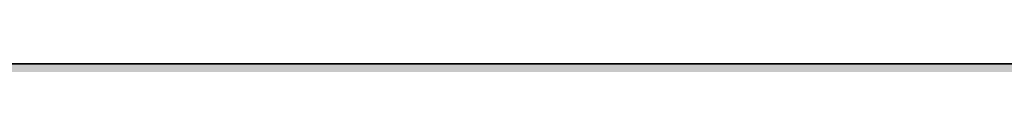
# Model space of a CAD drawing. Units: inches. Extents: x 2091 to 2899, y 967 to 2217.
# Tile 83 of 256: x 2249.731 to 2251.243, y 1099.919 to 1099.919. Entities that reach past the tile are written whole.
import ezdxf

# ---------------------------------------------------------------- set-up
doc = ezdxf.new("R2010")
doc.units = ezdxf.units.IN
doc.layers.add('A-WALL-PATT', color=141, linetype='Continuous', lineweight=13, true_color=0xadddf7)
doc.layers.add('L-SITE-WALL', color=7, linetype='Continuous', lineweight=35)

msp = doc.modelspace()

# ---------------------------------------------------------------- hatches: boundary and pattern name
at = {"layer": 'A-WALL-PATT'}
h = msp.add_hatch(color=256, dxfattribs=at)
h.dxf.hatch_style = 1
h.paths.add_polyline_path([(2212.1436, 1941.4191), (2387.6436, 1941.4191), (2387.6436, 1824.4191), (2392.1436, 1824.4191), (2392.1436, 1941.4191), (2609.6436, 1941.4191), (2609.6436, 1825.9191), (2614.1436, 1825.9191), (2614.1436, 1941.4191), (2794.1436, 1941.4191), (2794.1436, 1928.7622), (2803.1436, 1928.7622), (2803.1436, 2050.9191), (2203.1436, 2050.9191), (2203.1436, 1900.7579), (2212.1436, 1900.7579)])
h.paths.add_polyline_path([(2212.1436, 1945.9191), (2212.1436, 2041.9191), (2794.1436, 2041.9191), (2794.1436, 1945.9191), (2402.2482, 1945.9191), (2401.1024, 1945.7758), (2398.7024, 1945.7758)], flags=16)
h.paths.add_polyline_path([(2230.2299, 1948.0628), (2227.3499, 1949.5028), (2225.9099, 1951.9028), (2223.9899, 1952.8628), (2223.0299, 1955.2628), (2222.0699, 1959.5828), (2222.0699, 1963.4228), (2223.0299, 1965.6628), (2223.9899, 1965.3428), (2225.5859, 1963.8607), (2226.9115, 1964.9573), (2226.9489, 1965.9388), (2227.7783, 1966.9521), (2228.1999, 1968.8787), (2230.7099, 1964.8628), (2233.5899, 1966.3028), (2233.6073, 1966.3319), (2233.7727, 1964.9382), (2234.6338, 1963.6765), (2235.0299, 1963.9028), (2236.282, 1965.5724), (2235.9899, 1962.9428), (2237.9545, 1957.54), (2238.3899, 1957.9028), (2239.2159, 1960.3058), (2238.6546, 1966.385), (2238.6928, 1966.4381), (2238.8406, 1967.4997), (2238.7803, 1967.6875), (2238.8805, 1967.7868), (2238.6669, 1966.2518), (2239.2159, 1960.3058), (2238.3899, 1957.9028), (2236.9499, 1956.7028), (2234.5499, 1949.9828)], flags=0)
h.paths.add_polyline_path([(2278.012, 1948.0628), (2276.4964, 1947.8733), (2275.8498, 1947.6886), (2274.652, 1947.1028)], flags=0)
h.paths.add_polyline_path([(2269.852, 1955.7428), (2268.2762, 1956.6293), (2270.8673, 1956.3484), (2269.372, 1958.1428), (2268.715, 1959.1923), (2270.5698, 1958.7286), (2268.5807, 1961.9061), (2270.812, 1960.8919), (2270.812, 1963.4228), (2271.3933, 1964.7793), (2270.2918, 1966.1562), (2271.772, 1965.6628), (2272.1414, 1966.5248), (2273.9298, 1965.9286), (2275.6304, 1968.0543), (2276.3319, 1966.7219), (2276.5204, 1966.9521), (2276.942, 1968.8787), (2277.7343, 1967.6111), (2278.1399, 1969.4645), (2279.6591, 1967.0337), (2280.412, 1966.7828), (2280.9493, 1967.5888), (2281.6098, 1967.3686), (2282.1333, 1968.1538), (2282.3492, 1966.3334), (2282.3498, 1966.3326), (2283.4076, 1968.0954), (2283.7126, 1965.524), (2284.3202, 1964.6338), (2284.5118, 1964.8892), (2284.235, 1965.7048), (2284.5005, 1967.319), (2284.9079, 1965.4174), (2285.3963, 1966.0686), (2285.4328, 1966.2906), (2285.4733, 1966.1713), (2286.3539, 1967.3454), (2286.222, 1966.1582), (2287.6635, 1968.0802), (2287.714, 1968.4428), (2288.4816, 1969.0167), (2288.574, 1968.7289), (2288.9175, 1969.069), (2288.6068, 1966.8376), (2288.9287, 1963.3513), (2288.935, 1963.3568), (2288.9297, 1963.3404), (2289.0153, 1962.4139), (2290.1112, 1963.8751), (2290.1328, 1963.9426), (2290.2177, 1964.0171), (2290.1112, 1963.8751), (2289.1558, 1960.8916), (2288.594, 1959.2572), (2288.572, 1959.1028), (2289.532, 1960.5428), (2290.012, 1962.4628), (2290.1918, 1962.6427), (2289.7698, 1959.6886), (2286.8898, 1957.2886), (2284.4898, 1950.5686), (2283.3147, 1950.0463), (2283.292, 1949.9828), (2280.2901, 1948.6486), (2281.1298, 1948.6486), (2282.5698, 1948.1686), (2283.2047, 1948.0628), (2278.972, 1948.0628), (2276.092, 1949.5028), (2274.652, 1951.9028), (2272.732, 1952.8628)], flags=0)
h.paths.add_polyline_path([(2271.1589, 1958.0218), (2272.9698, 1955.8486), (2272.0098, 1960.1686), (2272.0098, 1964.0086), (2272.6244, 1965.4427), (2274.328, 1963.8607), (2275.6536, 1964.9573), (2275.6377, 1964.5391), (2277.4122, 1966.0069), (2277.033, 1965.1568), (2276.8299, 1964.9756), (2276.766, 1963.295), (2277.4496, 1962.6602), (2279.452, 1964.8628), (2282.332, 1966.3028), (2283.5298, 1966.8886), (2283.2945, 1966.7709), (2283.913, 1963.8847), (2284.8992, 1964.4483), (2284.732, 1962.9428), (2286.6966, 1957.54), (2287.132, 1957.9028), (2287.5419, 1959.0954), (2287.7794, 1958.4423), (2285.6827, 1956.6951), (2285.8765, 1959.7953), (2284.732, 1962.9428), (2284.8992, 1964.4483), (2283.913, 1963.8847), (2284.2238, 1962.4341), (2283.4244, 1963.6055), (2281.6098, 1962.5686), (2281.1298, 1960.1686), (2282.0898, 1956.3286), (2283.0498, 1952.9686), (2282.5698, 1950.5686), (2280.1698, 1948.6486), (2279.8833, 1948.7919), (2278.972, 1948.0628), (2278.972, 1949.0228), (2278.6723, 1949.3974), (2277.2898, 1950.0886), (2275.8498, 1952.4886), (2273.9298, 1953.4486), (2272.4898, 1954.8886), (2271.9216, 1954.8886), (2271.772, 1955.2628)], flags=0)
h.paths.add_polyline_path([(2311.9941, 1955.7428), (2312.0627, 1955.6742), (2312.0551, 1955.7085)], flags=0)
h.paths.add_polyline_path([(2331.9561, 1963.9518), (2333.3961, 1965.3918), (2331.0771, 1963.3568), (2330.9986, 1963.1115)], flags=0)
h.paths.add_polyline_path([(2310.5541, 1954.3028), (2307.0398, 1956.2799), (2310.7629, 1955.8763), (2312.4741, 1953.8228), (2313.4341, 1951.4228), (2315.3541, 1950.4628), (2316.7941, 1948.0628), (2317.4661, 1947.7268), (2319.3687, 1947.9646), (2317.7541, 1949.9828), (2317.5695, 1950.6105), (2316.7941, 1951.9028), (2314.8741, 1952.8628), (2313.9141, 1955.2628), (2311.5141, 1958.1428), (2309.3755, 1961.5592), (2311.5141, 1960.3371), (2311.5141, 1961.9828), (2310.6047, 1963.1196), (2311.7266, 1962.4785), (2312.4183, 1964.0926), (2312.256, 1964.2955), (2313.1941, 1963.9828), (2313.9141, 1965.6628), (2314.6468, 1965.4186), (2315.3541, 1966.3028), (2316.7941, 1967.7428), (2316.1574, 1966.9469), (2317.0341, 1965.2819), (2317.2226, 1965.5121), (2317.777, 1968.0458), (2318.4741, 1966.7219), (2318.6626, 1966.9521), (2319.0842, 1968.8787), (2321.207, 1965.4821), (2322.1614, 1966.9137), (2322.5541, 1966.7828), (2322.786, 1967.1306), (2322.8816, 1966.3243), (2323.312, 1965.7217), (2323.6513, 1965.8914), (2324.3965, 1967.1334), (2324.6569, 1964.9382), (2324.972, 1964.4766), (2325.3873, 1967.0015), (2325.9408, 1964.4183), (2327.2289, 1966.1358), (2327.1663, 1965.5724), (2328.0591, 1966.7628), (2328.2246, 1966.2475), (2329.668, 1967.6769), (2329.6646, 1967.6875), (2329.7648, 1967.7868), (2329.5511, 1966.2518), (2330.1001, 1960.3058), (2329.3328, 1958.0735), (2329.3131, 1957.9352), (2329.6341, 1958.2028), (2330.2341, 1959.1028), (2330.7141, 1961.0228), (2331.0341, 1961.3428), (2330.7141, 1959.1028), (2329.6341, 1958.2028), (2329.2741, 1957.6628), (2327.7121, 1956.3611), (2325.4341, 1949.9828), (2324.3338, 1949.4937), (2323.9941, 1948.5428), (2319.6741, 1946.6228), (2316.7941, 1948.0628), (2315.3541, 1950.4628), (2313.4341, 1951.4228)], flags=0)
h.paths.add_polyline_path([(2321.3357, 1947.952), (2321.1141, 1948.0628), (2321.1141, 1949.0228), (2319.1941, 1951.4228), (2316.7941, 1959.5828), (2316.6632, 1959.5828), (2315.3541, 1958.1428), (2314.3941, 1958.1428), (2313.1483, 1958.7091), (2312.9541, 1959.5828), (2312.9541, 1960.8919), (2315.8341, 1959.5828), (2316.6632, 1959.5828), (2317.3147, 1960.2994), (2315.0302, 1962.4207), (2316.3558, 1963.5173), (2316.3723, 1963.9516), (2316.4702, 1963.8607), (2317.7958, 1964.9573), (2317.7552, 1963.8897), (2319.1751, 1965.1568), (2319.4984, 1965.8814), (2321.1141, 1965.3428), (2323.2359, 1962.3724), (2325.6863, 1963.7726), (2325.5428, 1962.4806), (2325.1988, 1963.494), (2324.4785, 1963.0824), (2324.926, 1960.9941), (2324.0781, 1962.2365), (2322.4148, 1961.286), (2322.0741, 1959.5828), (2323.0341, 1955.7428), (2323.9941, 1952.3828), (2323.5141, 1949.9828), (2322.1427, 1948.8856), (2322.0741, 1948.5428)], flags=0)
h.paths.add_polyline_path([(2320.2075, 1963.3375), (2320.1541, 1963.4228), (2320.3941, 1963.5428)], flags=0)
h.paths.add_polyline_path([(2353.8505, 1965.8105), (2354.0305, 1965.7505), (2354.3305, 1966.4505), (2354.3305, 1966.9305)], flags=0)
h.paths.add_polyline_path([(2359.0206, 1969.0264), (2359.0984, 1968.9019), (2359.2335, 1969.5195), (2359.2335, 1969.9995)], flags=0)
h.paths.add_polyline_path([(2358.2567, 1966.6817), (2357.9836, 1966.348), (2358.2113, 1966.1462), (2358.4105, 1966.3896)], flags=0)
h.paths.add_polyline_path([(2357.7685, 1966.0588), (2357.7322, 1965.105), (2357.751, 1965.1206), (2357.7695, 1965.6065), (2357.7695, 1966.0578)], flags=0)
h.paths.add_polyline_path([(2359.1115, 1965.3045), (2359.1115, 1964.8245), (2359.8445, 1966.4675), (2359.8445, 1966.9475)], flags=0)
h.paths.add_polyline_path([(2360.2237, 1966.6214), (2360.6985, 1969.3625), (2360.6985, 1969.8425), (2360.2105, 1967.0255), (2360.2105, 1966.6425)], flags=0)
h.paths.add_polyline_path([(2363.4505, 1967.8905), (2363.4505, 1968.3705), (2362.4905, 1966.9305), (2362.656, 1966.6988)], flags=0)
h.paths.add_polyline_path([(2364.4755, 1966.0788), (2365.8505, 1968.3705), (2365.8505, 1968.8505), (2364.428, 1966.4796)], flags=0)
h.paths.add_polyline_path([(2366.3135, 1965.8525), (2366.3667, 1965.6958), (2366.8025, 1968.3455), (2366.8025, 1968.8255)], flags=0)
h.paths.add_polyline_path([(2367.1653, 1965.8035), (2367.2905, 1966.9305), (2367.2905, 1967.4105), (2367.1027, 1965.7201)], flags=0)
h.paths.add_polyline_path([(2370.0365, 1959.9735), (2371.0135, 1963.0245), (2371.0135, 1963.5045), (2370.0365, 1960.4535)], flags=0)
h.paths.add_polyline_path([(2371.6105, 1960.2105), (2372.5705, 1961.6505), (2372.5705, 1962.1305), (2371.8025, 1960.9785)], flags=0)
h.paths.add_polyline_path([(2350.8737, 1956.0051), (2351.9305, 1955.8905), (2354.4905, 1953.3305), (2353.8505, 1954.9305), (2351.4505, 1957.8105), (2347.9355, 1963.4255), (2347.9355, 1963.9055), (2351.4505, 1958.2905), (2353.7051, 1955.585), (2352.8905, 1959.2505), (2352.8905, 1959.7305), (2352.8905, 1961.9248), (2356.7305, 1959.7305), (2358.4545, 1961.6268), (2354.8105, 1965.0105), (2355.0309, 1965.2859), (2358.6911, 1961.8871), (2361.5305, 1965.0105), (2364.3765, 1966.4335), (2364.5244, 1965.1869), (2365.4545, 1963.8242), (2365.8811, 1964.068), (2365.3705, 1966.4505), (2365.3705, 1966.9305), (2366.8105, 1960.2105), (2366.8105, 1959.7305), (2366.3887, 1952.9814), (2367.7705, 1956.8505), (2368.6412, 1957.5761), (2366.8105, 1962.6105), (2366.8105, 1963.0905), (2368.7752, 1957.6877), (2369.2105, 1958.0505), (2370.0016, 1960.3519), (2369.4752, 1966.0527), (2369.5135, 1966.1058), (2369.5142, 1966.1109), (2369.4752, 1966.5327), (2369.5135, 1966.5858), (2369.6146, 1967.3126), (2369.1825, 1968.6585), (2369.1825, 1969.1385), (2369.601, 1967.8352), (2369.7012, 1967.9345), (2369.7179, 1968.0547), (2370.1452, 1968.3741), (2369.7787, 1968.0112), (2369.7012, 1967.4545), (2370.4682, 1968.214), (2369.6749, 1967.2658), (2369.5142, 1966.1109), (2370.0365, 1960.4535), (2370.0365, 1959.9735), (2369.4418, 1958.2432), (2370.6505, 1959.2505), (2371.0458, 1962.0176), (2371.1305, 1962.1305), (2370.6505, 1958.7705), (2367.7705, 1956.3705), (2365.3705, 1949.6505), (2362.0791, 1948.1876), (2363.4505, 1947.7305), (2361.0505, 1947.7305), (2360.0905, 1947.7305), (2357.1039, 1947.3572), (2360.0905, 1948.2105), (2358.1705, 1949.1705), (2356.7305, 1951.5705), (2354.8105, 1952.5305), (2351.9305, 1955.4105)], flags=0)
h.paths.add_polyline_path([(2361.0505, 1948.6905), (2359.1305, 1951.0905), (2356.7305, 1959.2505), (2355.7705, 1959.2505), (2352.8905, 1960.5596), (2352.8905, 1961.4448), (2355.8905, 1959.7305), (2356.7305, 1959.7305), (2356.8372, 1959.3678), (2361.5305, 1964.5305), (2363.2484, 1965.3894), (2364.9253, 1963.0418), (2362.4905, 1961.6505), (2362.0639, 1959.5172), (2362.9705, 1955.8905), (2363.9305, 1952.5305), (2363.9305, 1952.0505), (2363.4505, 1949.6505), (2361.0505, 1947.7305)], flags=0)
h.paths.add_polyline_path([(2359.1305, 1951.5705), (2359.2905, 1951.3705), (2361.0505, 1954.4505), (2361.0505, 1954.9305)], flags=0)
h.paths.add_polyline_path([(2357.2195, 1966.5455), (2356.7925, 1968.8145), (2356.7925, 1969.2945), (2357.2195, 1967.0255)], flags=0)
h.paths.add_polyline_path([(2361.0505, 1954.4505), (2361.5305, 1958.7705), (2361.5305, 1959.2505), (2361.0505, 1954.9305)], flags=0)
h.paths.add_polyline_path([(2402.5483, 1948.4861), (2402.3024, 1948.4158), (2402.5904, 1948.4158)], flags=0)
h.paths.add_polyline_path([(2394.1424, 1956.0958), (2395.6851, 1954.5532), (2396.7205, 1953.9707), (2396.0624, 1955.6158), (2395.2414, 1956.6011), (2395.8789, 1956.4417), (2395.1024, 1959.9358), (2395.1024, 1963.7758), (2396.0624, 1966.0158), (2397.0224, 1965.6958), (2398.6185, 1964.2138), (2399.9441, 1965.3103), (2399.9814, 1966.2918), (2400.8109, 1967.3052), (2401.2325, 1969.2317), (2403.5379, 1965.543), (2403.942, 1967.3893), (2404.7024, 1967.1358), (2405.4603, 1966.0748), (2406.6224, 1966.6558), (2406.6399, 1966.6849), (2406.8052, 1965.2912), (2406.9257, 1965.1147), (2407.3424, 1964.9758), (2407.8743, 1965.7737), (2408.1691, 1964.3981), (2409.3146, 1965.9254), (2409.2175, 1965.0511), (2409.4452, 1963.1312), (2410.3064, 1961.8695), (2410.7024, 1962.0958), (2411.4423, 1963.0823), (2411.1654, 1963.8978), (2411.6164, 1966.6398), (2411.7254, 1966.7911), (2411.8732, 1967.8527), (2411.8129, 1968.0405), (2411.9131, 1968.1398), (2411.6994, 1966.6048), (2412.2484, 1960.6588), (2413.2254, 1963.7098), (2414.3779, 1964.7212), (2414.5132, 1965.6927), (2414.4529, 1965.8805), (2414.5531, 1965.9798), (2414.3779, 1964.7212), (2414.5198, 1964.8457), (2414.3654, 1964.6311), (2414.3394, 1964.4448), (2414.8884, 1958.4988), (2414.0624, 1956.0958), (2412.6224, 1954.8958), (2410.1714, 1948.0329), (2410.0167, 1948.0844), (2405.9024, 1946.2558), (2405.9024, 1947.2158), (2405.2043, 1948.0886), (2404.2224, 1948.4158), (2403.2624, 1948.4158), (2400.3824, 1949.8558), (2399.6624, 1951.0558), (2397.9824, 1952.7358), (2397.0224, 1953.2158), (2395.6851, 1954.5532), (2392.6568, 1956.2569)], flags=0)
h.paths.add_polyline_path([(2409.0857, 1964.4074), (2409.1304, 1964.2757), (2409.2624, 1964.4958)], flags=0)
h.paths.add_polyline_path([(2397.7424, 1961.6158), (2398.7024, 1963.8558), (2399.6624, 1963.5358), (2401.4266, 1965.741), (2401.7914, 1966.5588), (2402.0714, 1965.0708), (2402.8355, 1964.3934), (2403.2624, 1964.9149), (2403.3381, 1964.7711), (2402.6155, 1963.9762), (2402.4986, 1960.9022), (2403.543, 1959.9325), (2404.4132, 1960.8897), (2404.7024, 1962.3358), (2407.9163, 1964.1724), (2409.5202, 1961.9269), (2410.9871, 1957.893), (2411.4224, 1958.2558), (2412.048, 1960.0756), (2412.4103, 1959.0791), (2411.6756, 1958.4668), (2411.6624, 1958.2558), (2411.6261, 1958.4255), (2409.9824, 1957.0558), (2407.5824, 1950.3358), (2403.2624, 1948.4158), (2403.2624, 1949.3758), (2401.3424, 1951.7758), (2399.4165, 1958.324), (2397.7424, 1959.0849), (2397.7424, 1959.9701), (2397.1024, 1960.3358), (2397.7424, 1960.0449)], flags=0)
h.paths.add_polyline_path([(2405.9024, 1952.9758), (2405.9504, 1953.4078), (2406.0167, 1953.1758)], flags=0)
h.paths.add_polyline_path([(2449.8178, 1967.114), (2449.7523, 1967.1358), (2449.7937, 1967.0779)], flags=0)
h.paths.add_polyline_path([(2451.6977, 1966.6181), (2451.7409, 1966.6901), (2451.6921, 1966.6657)], flags=0)
h.paths.add_polyline_path([(2454.3436, 1965.7376), (2455.7523, 1967.6158), (2455.9923, 1968.0958), (2454.3645, 1965.9254)], flags=0)
h.paths.add_polyline_path([(2457.5473, 1968.8638), (2457.7873, 1969.3438), (2457.0543, 1968.7958), (2457.0076, 1968.4603)], flags=0)
h.paths.add_polyline_path([(2456.9218, 1967.8567), (2456.8022, 1968.229), (2456.723, 1967.6598)], flags=0)
h.paths.add_polyline_path([(2457.3023, 1967.3768), (2457.5423, 1967.8568), (2456.8103, 1966.8398), (2456.7405, 1966.7002), (2456.749, 1966.6081)], flags=0)
h.paths.add_polyline_path([(2458.2753, 1963.7098), (2458.1553, 1963.3352), (2460.3543, 1965.2648), (2460.5943, 1965.7448)], flags=0)
h.paths.add_polyline_path([(2458.3923, 1962.8158), (2458.3641, 1962.6182), (2459.5923, 1964.2558), (2459.8323, 1964.7358)], flags=0)
h.paths.add_polyline_path([(2459.3523, 1962.8158), (2459.2723, 1962.4958), (2460.0723, 1963.2958), (2460.3123, 1963.7758)], flags=0)
h.paths.add_polyline_path([(2458.6803, 1960.6078), (2458.6323, 1960.4158), (2459.5923, 1961.8558), (2459.8323, 1962.3358)], flags=0)
h.paths.add_polyline_path([(2437.8382, 1956.2427), (2439.1923, 1956.0958), (2441.3523, 1953.9358), (2440.8723, 1955.1358), (2438.4723, 1958.0158), (2438.0716, 1958.656), (2438.7123, 1958.4958), (2440.6396, 1956.1831), (2439.9123, 1959.4558), (2439.9123, 1963.2958), (2441.3523, 1966.6558), (2441.5923, 1967.1358), (2441.1123, 1966.0158), (2442.0723, 1965.6958), (2443.989, 1968.0917), (2444.2413, 1966.7508), (2444.9168, 1966.1519), (2445.6766, 1967.0801), (2446.2553, 1969.7248), (2446.4953, 1970.2048), (2446.2824, 1969.2317), (2447.3627, 1967.5033), (2447.7203, 1969.5678), (2447.9603, 1970.0478), (2447.4855, 1967.3068), (2448.7923, 1965.2158), (2448.4723, 1964.8638), (2448.5523, 1964.7358), (2451.4521, 1966.1857), (2451.6151, 1964.8112), (2452.3079, 1963.7962), (2453.2345, 1964.3257), (2454.0723, 1960.4158), (2453.6287, 1953.3177), (2454.7923, 1956.5758), (2455.0323, 1957.0558), (2455.7188, 1957.6279), (2453.8323, 1962.8158), (2453.941, 1963.7936), (2453.3353, 1965.5778), (2453.8243, 1968.5508), (2454.0643, 1969.0308), (2453.5753, 1966.0578), (2454.0403, 1964.6879), (2453.8323, 1962.8158), (2455.7188, 1957.6279), (2456.3672, 1958.1682), (2457.0583, 1960.1788), (2457.2983, 1960.6588), (2456.4723, 1958.2558), (2457.7177, 1959.2937), (2457.6723, 1958.9758), (2454.89, 1956.6572), (2453.6141, 1953.0849), (2453.5923, 1952.7358), (2453.3523, 1952.2558), (2453.3596, 1952.3722), (2452.6323, 1950.3358), (2452.3923, 1949.8558), (2449.2038, 1948.4387), (2450.7123, 1947.9358), (2448.0723, 1947.9358), (2447.1123, 1947.9358), (2444.5523, 1947.6158), (2447.1996, 1948.3722), (2445.1923, 1949.3758), (2443.7523, 1951.7758), (2441.8323, 1952.7358), (2438.9523, 1955.6158)], flags=0)
h.paths.add_polyline_path([(2443.9923, 1959.9358), (2444.0403, 1959.7726), (2444.1216, 1959.862)], flags=0)
h.paths.add_polyline_path([(2442.9123, 1959.9358), (2443.0323, 1959.9358), (2442.4457, 1960.2025)], flags=0)
h.paths.add_polyline_path([(2444.9829, 1965.0197), (2445.2793, 1965.2648), (2445.5193, 1965.7448), (2444.994, 1965.3103)], flags=0)
h.paths.add_polyline_path([(2446.1333, 1965.0298), (2446.3304, 1965.4715), (2444.9703, 1964.2578), (2444.7303, 1963.7778)], flags=0)
h.paths.add_polyline_path([(2442.7923, 1959.4558), (2443.7523, 1959.4558), (2446.1523, 1951.2958), (2446.4123, 1951.7508), (2446.3923, 1951.7758), (2448.0806, 1954.7303), (2448.5523, 1958.9758), (2441.8323, 1965.2158), (2442.1549, 1965.6191), (2448.7923, 1959.4558), (2448.3123, 1955.1358), (2448.0723, 1954.6558), (2446.4123, 1951.7508), (2448.3123, 1949.3758), (2448.3123, 1948.4158), (2450.5409, 1950.1987), (2450.9523, 1952.2558), (2449.9923, 1955.6158), (2449.0323, 1959.4558), (2449.5123, 1961.8558), (2449.7523, 1962.3358), (2449.6749, 1961.9487), (2452.9945, 1963.8457), (2453.0644, 1963.5194), (2452.8846, 1963.7829), (2449.6749, 1961.9487), (2449.2723, 1959.9358), (2450.2323, 1956.0958), (2451.1923, 1952.7358), (2450.7123, 1950.3358), (2450.4723, 1949.8558), (2448.0723, 1947.9358), (2448.0723, 1948.5358), (2445.4323, 1949.8558), (2443.9923, 1952.2558), (2442.0723, 1953.2158), (2441.1123, 1955.6158), (2440.1523, 1959.9358), (2440.1523, 1960.6558)], flags=0)
h.paths.add_polyline_path([(2456.6923, 1966.9858), (2457.6083, 1968.0808), (2457.8483, 1968.5608), (2456.9323, 1967.4658)], flags=0)
h.paths.add_polyline_path([(2489.8966, 1966.5802), (2489.9429, 1966.1893), (2490.7475, 1967.5302), (2491.3191, 1968.9512)], flags=0)
h.paths.add_polyline_path([(2473.5625, 1956.4071), (2477.14, 1956.0193), (2476.9553, 1956.2408), (2475.108, 1957.2801), (2476.3475, 1956.9702), (2475.1869, 1958.8242), (2476.9191, 1958.3912), (2475.4116, 1960.7993), (2477.7875, 1959.7193), (2477.7875, 1962.2502), (2477.6374, 1962.4379), (2477.8226, 1962.3321), (2478.3591, 1963.5841), (2478.3591, 1963.6712), (2477.3243, 1964.9646), (2478.7148, 1964.5011), (2479.3191, 1965.9112), (2480.2791, 1965.5912), (2481.784, 1967.4722), (2482.1165, 1965.7052), (2482.8806, 1965.0278), (2483.2093, 1965.4294), (2483.2202, 1965.7151), (2483.0759, 1965.989), (2483.7118, 1966.7658), (2484.1305, 1968.6792), (2484.7021, 1970.1002), (2484.4892, 1969.1271), (2486.5029, 1965.9051), (2487.3875, 1965.6102), (2488.1534, 1966.7591), (2488.717, 1965.9701), (2489.2001, 1966.2116), (2489.3307, 1965.111), (2490.3939, 1963.6225), (2490.6608, 1963.775), (2490.4939, 1964.5536), (2490.9231, 1963.9248), (2491.3191, 1964.1512), (2491.3334, 1964.1702), (2491.2105, 1964.5322), (2491.2818, 1964.9655), (2491.4258, 1964.2934), (2494.0765, 1967.8276), (2494.4979, 1966.5149), (2494.5982, 1966.6142), (2494.6895, 1967.2702), (2495.1067, 1967.5822), (2495.1298, 1967.7481), (2495.0696, 1967.9359), (2495.1698, 1968.0351), (2495.0318, 1967.0436), (2495.7538, 1967.7587), (2494.9821, 1966.6864), (2494.9561, 1966.5002), (2495.479, 1960.8369), (2495.9105, 1962.1842), (2496.4821, 1963.6052), (2496.0727, 1962.3266), (2496.7689, 1962.9375), (2496.5991, 1962.7112), (2496.1191, 1959.3512), (2496.7329, 1960.2718), (2496.9875, 1961.2902), (2497.5591, 1962.7112), (2497.0791, 1960.7912), (2496.5075, 1959.3702), (2495.5475, 1957.9302), (2492.7588, 1955.6064), (2490.8391, 1950.2312), (2490.2675, 1948.8102), (2485.9475, 1946.8902), (2483.0675, 1948.3302), (2481.6275, 1950.7302), (2479.7075, 1951.6902), (2476.8275, 1954.5702)], flags=0)
h.paths.add_polyline_path([(2485.577, 1948.3134), (2485.5591, 1948.3112), (2485.5788, 1948.3112)], flags=0)
h.paths.add_polyline_path([(2478.6451, 1954.5512), (2478.109, 1956.9633), (2479.3191, 1955.5112), (2480.2791, 1953.1112), (2482.1991, 1952.1512), (2483.6391, 1949.7512), (2486.5191, 1948.3112), (2486.5191, 1949.2712), (2484.7393, 1951.4959), (2484.0275, 1950.2502), (2481.6275, 1958.4102), (2482.3751, 1959.2327), (2482.1991, 1959.8312), (2483.1976, 1960.9295), (2479.7075, 1964.1702), (2480.6034, 1965.2901), (2481.8752, 1964.1091), (2482.6664, 1964.7636), (2482.6154, 1963.4218), (2482.9892, 1963.0747), (2484.0085, 1963.9842), (2484.6836, 1965.4975), (2484.5801, 1965.4052), (2485.3573, 1967.1471), (2485.1206, 1965.7812), (2486.4275, 1963.6902), (2488.1454, 1964.5492), (2489.8223, 1962.2016), (2490.7475, 1962.7302), (2491.9997, 1964.3998), (2492.076, 1965.0873), (2492.2129, 1964.6841), (2492.4854, 1965.0474), (2492.2791, 1963.1912), (2494.2438, 1957.7884), (2494.5625, 1958.054), (2494.9335, 1959.1332), (2495.5051, 1960.5542), (2494.6791, 1958.1512), (2494.1075, 1956.7302), (2494.5625, 1958.054), (2493.4085, 1957.0923), (2491.7075, 1961.7702), (2491.9997, 1964.3998), (2490.7475, 1962.7302), (2487.712, 1960.9957), (2487.4791, 1959.8312), (2488.4391, 1955.9912), (2489.3991, 1952.6312), (2488.9191, 1950.2312), (2488.5769, 1949.9574), (2488.3475, 1948.8102), (2487.6517, 1948.2536), (2487.4791, 1948.3112), (2486.5191, 1948.3112), (2483.6391, 1949.7512), (2482.1991, 1952.1512), (2480.2791, 1953.1112), (2478.8391, 1954.5512)], flags=0)
h.paths.add_polyline_path([(2526.6483, 1966.9875), (2526.5173, 1967.0312), (2526.6001, 1966.9153)], flags=0)
h.paths.add_polyline_path([(2528.4706, 1966.4467), (2528.5745, 1966.6197), (2528.4571, 1966.561)], flags=0)
h.paths.add_polyline_path([(2534.1333, 1967.4962), (2534.1567, 1967.5428), (2534.0598, 1967.4083)], flags=0)
h.paths.add_polyline_path([(2536.1619, 1964.0506), (2535.1573, 1962.7112), (2535.1009, 1962.3159), (2536.1173, 1963.6712), (2536.4205, 1964.2775)], flags=0)
h.paths.add_polyline_path([(2535.1573, 1959.8312), (2536.1173, 1961.2712), (2536.5973, 1962.2312), (2535.2533, 1960.2152)], flags=0)
h.paths.add_polyline_path([(2513.249, 1956.2848), (2516.2212, 1955.9626), (2514.9973, 1957.4312), (2514.1958, 1958.7115), (2515.4773, 1958.3912), (2516.9319, 1956.6457), (2516.4373, 1958.8712), (2516.4373, 1962.7112), (2516.8727, 1963.727), (2515.3464, 1965.6348), (2517.3973, 1964.9512), (2517.8773, 1966.0712), (2518.3573, 1967.0312), (2517.8773, 1965.9112), (2518.8373, 1965.5912), (2520.4866, 1967.6527), (2520.7663, 1966.1662), (2521.5304, 1965.4887), (2521.7814, 1965.7954), (2521.8009, 1966.3073), (2521.4778, 1966.9209), (2521.2463, 1967.1262), (2521.1777, 1967.4909), (2521.4778, 1966.9209), (2522.0104, 1966.4487), (2522.2574, 1966.7504), (2522.7803, 1969.1402), (2523.2603, 1970.1002), (2523.0474, 1969.1271), (2524.6731, 1966.5259), (2526.0373, 1966.0712), (2526.7952, 1965.0101), (2527.9771, 1965.601), (2528.1401, 1964.2266), (2528.6646, 1963.4582), (2529.3886, 1963.8719), (2529.3297, 1964.147), (2529.4813, 1963.9248), (2529.8773, 1964.1512), (2529.984, 1964.2934), (2529.7891, 1965.2032), (2530.0624, 1964.3979), (2532.8025, 1968.0513), (2533.1478, 1966.9759), (2533.248, 1967.0751), (2533.3393, 1967.7312), (2533.6728, 1967.9805), (2533.728, 1968.0351), (2533.5143, 1966.5002), (2534.0247, 1960.9725), (2534.5603, 1962.6452), (2535.0403, 1963.6052), (2534.0633, 1960.5542), (2533.2373, 1958.1512), (2534.2882, 1959.0268), (2534.1973, 1958.3912), (2531.5126, 1956.1539), (2529.3973, 1950.2312), (2528.9173, 1949.2712), (2526.4488, 1948.174), (2527.4773, 1947.8312), (2530.3573, 1947.3512), (2524.5973, 1947.3512), (2521.7173, 1948.7912), (2520.2773, 1951.1912), (2518.3573, 1952.1512), (2515.4773, 1955.0312)], flags=0)
h.paths.add_polyline_path([(2523.9348, 1967.1903), (2523.6195, 1966.4837), (2523.7705, 1966.2421)], flags=0)
h.paths.add_polyline_path([(2518.8373, 1953.1112), (2517.8773, 1955.5112), (2516.885, 1959.9768), (2516.9173, 1959.9621), (2516.9173, 1962.0254), (2520.7573, 1959.8312), (2522.0249, 1961.2255), (2518.3573, 1964.6312), (2519.0026, 1965.4377), (2520.4334, 1964.1091), (2521.3011, 1964.8269), (2521.2452, 1963.3553), (2525.6383, 1959.276), (2526.0373, 1961.2712), (2529.3973, 1963.1912), (2530.6495, 1964.8607), (2530.6647, 1964.9976), (2530.692, 1964.9173), (2531.0878, 1965.4451), (2530.946, 1964.1689), (2530.692, 1964.9173), (2529.3973, 1963.1912), (2526.3625, 1961.457), (2526.0373, 1959.8312), (2526.9973, 1955.9912), (2527.9573, 1952.6312), (2527.4773, 1950.2312), (2527.1345, 1949.9569), (2526.9739, 1949.1541), (2526.6973, 1949.0312), (2524.5973, 1947.3512), (2524.5973, 1948.3112), (2524.2773, 1948.7112), (2522.1973, 1949.7512), (2520.7573, 1952.1512)], flags=0)
h.paths.add_polyline_path([(2520.2773, 1958.8712), (2520.8533, 1959.5048), (2523.1573, 1951.6712), (2524.6139, 1954.2201), (2524.5973, 1954.0712), (2522.6773, 1950.7112)], flags=0)
h.paths.add_polyline_path([(2559.3709, 1966.3112), (2559.3984, 1966.3249), (2559.4019, 1966.3453)], flags=0)
h.paths.add_polyline_path([(2549.7709, 1957.1912), (2552.6509, 1954.3112), (2552.134, 1955.6035), (2550.6109, 1957.4312), (2547.0959, 1963.0462), (2545.7759, 1965.2062), (2549.2909, 1959.5912), (2551.6909, 1956.7112), (2550.7929, 1960.7521), (2550.7309, 1960.7803), (2550.7309, 1964.8712), (2551.6909, 1967.1112), (2552.6509, 1966.7912), (2554.247, 1965.3091), (2555.0343, 1965.9603), (2555.5817, 1966.6446), (2555.6099, 1967.3872), (2556.4394, 1968.4005), (2556.861, 1970.3271), (2559.3709, 1966.3112), (2560.6909, 1964.1512), (2562.4088, 1965.0101), (2561.6509, 1966.0712), (2560.3309, 1968.2312), (2561.7585, 1966.2325), (2562.3472, 1967.1156), (2562.4337, 1966.3866), (2563.1278, 1965.3696), (2563.5709, 1965.5912), (2563.5884, 1965.6202), (2563.3625, 1967.5235), (2563.7225, 1965.8438), (2565.06, 1968.073), (2564.7329, 1965.1287), (2565.1176, 1963.3334), (2567.4446, 1966.4361), (2567.3156, 1967.8333), (2567.3538, 1967.8864), (2567.5016, 1968.9481), (2567.4413, 1969.1359), (2567.5416, 1969.2351), (2567.3279, 1967.7002), (2567.8769, 1961.7542), (2568.7467, 1964.4703), (2568.6356, 1965.6733), (2568.6738, 1965.7264), (2568.8216, 1966.7881), (2568.7613, 1966.9759), (2568.8616, 1967.0751), (2568.6479, 1965.5402), (2568.7261, 1964.693), (2568.8539, 1964.8052), (2568.7467, 1964.4703), (2568.8172, 1963.7063), (2568.9709, 1963.9112), (2568.8661, 1963.1773), (2569.1969, 1959.5942), (2568.3709, 1957.1912), (2566.9309, 1955.9912), (2564.6203, 1949.5214), (2564.6509, 1949.5112), (2564.6166, 1949.5112), (2564.5309, 1949.2712), (2560.2109, 1947.3512), (2557.3309, 1948.7912), (2556.0452, 1950.934), (2556.0109, 1950.9512), (2555.8566, 1951.2083), (2553.9709, 1952.1512), (2551.0909, 1955.0312), (2546.6501, 1957.5295)], flags=0)
h.paths.add_polyline_path([(2567.0258, 1959.3302), (2567.035, 1959.3049), (2567.0509, 1959.3512)], flags=0)
h.paths.add_polyline_path([(2551.9683, 1962.5184), (2553.0109, 1964.9512), (2553.9709, 1964.6312), (2555.567, 1963.1491), (2556.8926, 1964.2456), (2556.9299, 1965.2272), (2557.144, 1965.4887), (2556.4201, 1966.1306), (2556.3914, 1966.105), (2556.3799, 1966.1662), (2556.4201, 1966.1306), (2556.9519, 1966.6052), (2557.0921, 1966.9195), (2557.5709, 1966.0102), (2557.7594, 1966.2405), (2557.4179, 1964.6802), (2556.8926, 1964.2456), (2556.8071, 1961.9976), (2560.6909, 1958.3912), (2560.6355, 1957.8927), (2560.8109, 1957.1912), (2561.7709, 1953.8312), (2561.2909, 1951.4312), (2559.1104, 1949.6868), (2559.1565, 1949.6292), (2563.0265, 1951.3492), (2562.6109, 1949.2712), (2560.2109, 1947.3512), (2560.2109, 1948.3112), (2559.2509, 1949.5112), (2558.8909, 1949.5112), (2558.8909, 1949.9612), (2558.2909, 1950.7112), (2558.0537, 1951.5177), (2556.9709, 1952.8712), (2555.0679, 1959.3415), (2552.0509, 1961.0654), (2552.0509, 1962.4712)], flags=0)
h.paths.add_polyline_path([(2588.33, 1958.3912), (2588.6102, 1958.111), (2588.5534, 1958.3669)], flags=0)
h.paths.add_polyline_path([(2594.7455, 1950.4931), (2593.9575, 1953.172), (2593.13, 1954.5512), (2591.21, 1955.5112), (2590.25, 1957.9112), (2588.309, 1960.2404), (2586.1773, 1961.2093), (2587.85, 1960.7912), (2587.2534, 1961.7442), (2588.4413, 1961.0654), (2588.4413, 1962.6555), (2588.4217, 1962.6653), (2588.4413, 1962.7112), (2586.914, 1964.6203), (2588.8771, 1963.728), (2589.29, 1964.6915), (2589.29, 1966.0712), (2590.25, 1968.3112), (2591.21, 1967.9912), (2592.8061, 1966.5091), (2594.1317, 1967.6056), (2594.169, 1968.5872), (2594.9985, 1969.6005), (2595.4201, 1971.5271), (2597.93, 1967.5112), (2600.81, 1968.9512), (2600.8275, 1968.9802), (2600.9928, 1967.5866), (2601.854, 1966.3248), (2602.1071, 1966.4695), (2602.2364, 1967.2551), (2602.3567, 1966.6934), (2603.5022, 1968.2207), (2603.21, 1965.5912), (2605.1747, 1960.1884), (2605.5069, 1960.4652), (2605.026, 1965.6733), (2605.0642, 1965.7264), (2605.212, 1966.7881), (2605.1517, 1966.9759), (2605.252, 1967.0751), (2605.3433, 1967.7312), (2605.9529, 1968.1869), (2605.8748, 1969.0333), (2605.913, 1969.0864), (2606.0608, 1970.1481), (2606.0005, 1970.3359), (2606.1007, 1970.4351), (2605.887, 1968.9002), (2606.436, 1962.9542), (2605.61, 1960.5512), (2605.997, 1960.8737), (2606.5643, 1962.6452), (2608.2415, 1964.1169), (2608.01, 1963.1912), (2607.05, 1961.7512), (2606.6315, 1961.4024), (2606.2013, 1958.3912), (2603.3213, 1955.9912), (2600.9213, 1949.2712), (2596.6013, 1947.3512), (2593.7213, 1948.7912), (2592.8573, 1950.2312), (2592.65, 1950.2312)], flags=0)
h.paths.add_polyline_path([(2596.6013, 1947.3512), (2596.6013, 1948.3112), (2594.6813, 1950.7112), (2596.155, 1953.29), (2595.53, 1954.0712), (2593.1992, 1961.996), (2592.6513, 1962.5047), (2591.7802, 1963.0025), (2593.283, 1964.2456), (2593.3203, 1965.2272), (2594.1498, 1966.2405), (2594.5714, 1968.1671), (2596.1827, 1965.589), (2596.9513, 1966.4345), (2598.0413, 1966.0712), (2598.7992, 1965.0101), (2599.9613, 1965.5912), (2599.9788, 1965.6202), (2600.1441, 1964.2266), (2601.0053, 1962.9648), (2601.4013, 1963.1912), (2602.6535, 1964.8607), (2602.3613, 1962.2312), (2603.7927, 1958.2947), (2601.9776, 1953.2124), (2601.9462, 1952.7095), (2599.4688, 1951.6084), (2599.0013, 1949.2712)], flags=0)
h.paths.add_polyline_path([(2597.5613, 1958.8712), (2597.671, 1959.4194), (2597.5951, 1958.7362)], flags=0)
h.paths.add_polyline_path([(2623.6663, 1961.2544), (2625.5192, 1960.7912), (2624.9655, 1961.6755), (2627.1992, 1960.6603), (2627.1992, 1961.1512), (2626.9592, 1962.2312), (2626.9592, 1963.4912), (2625.5823, 1965.2122), (2626.9592, 1964.4254), (2626.9592, 1965.8312), (2626.8692, 1965.8612), (2627.9192, 1968.3112), (2628.8792, 1967.9912), (2630.4752, 1966.5091), (2631.8008, 1967.6056), (2631.8382, 1968.5872), (2632.6676, 1969.6005), (2633.0892, 1971.5271), (2635.5992, 1967.5112), (2638.4792, 1968.9512), (2638.4966, 1968.9802), (2638.662, 1967.5866), (2639.1763, 1966.833), (2639.7802, 1967.8396), (2640.0258, 1966.6934), (2641.1713, 1968.2207), (2640.8792, 1965.5912), (2641.1143, 1964.9446), (2641.4113, 1965.3407), (2641.3081, 1964.4116), (2642.8438, 1960.1884), (2643.2792, 1960.5512), (2644.0847, 1962.8947), (2643.7839, 1966.1533), (2643.8068, 1966.1852), (2643.6007, 1968.4181), (2643.5228, 1968.6606), (2643.7299, 1970.1481), (2643.6696, 1970.3359), (2643.7698, 1970.4351), (2643.5562, 1968.9002), (2643.6007, 1968.4181), (2643.9096, 1967.4559), (2644.0098, 1967.5551), (2643.8117, 1966.1321), (2644.1052, 1962.9542), (2644.2388, 1961.3508), (2644.7192, 1961.7512), (2645.0329, 1962.2217), (2645.3222, 1963.1252), (2646.0764, 1963.787), (2645.0329, 1962.2217), (2644.3452, 1960.0742), (2643.5192, 1957.6712), (2642.0792, 1956.4712), (2639.7196, 1949.8644), (2639.8755, 1949.8384), (2635.3592, 1947.8312), (2632.4792, 1949.2712), (2631.0392, 1951.6712), (2629.1192, 1952.6312), (2628.1592, 1955.0312), (2625.7592, 1957.9112)], flags=0)
h.paths.add_polyline_path([(2627.8163, 1956.574), (2627.3737, 1958.5657), (2626.3763, 1959.7626), (2627.1992, 1959.3512), (2627.3737, 1958.5657), (2627.9192, 1957.9112), (2628.8792, 1955.5112), (2630.7992, 1954.5512), (2632.2392, 1952.1512), (2633.315, 1951.6132), (2631.0392, 1959.3512), (2631.4978, 1959.8557), (2630.7992, 1962.2312), (2631.4499, 1962.9469), (2630.7152, 1963.6291), (2632.0408, 1964.7256), (2632.0782, 1965.7072), (2632.2922, 1965.9687), (2631.7053, 1966.4891), (2633.1364, 1967.7661), (2633.3292, 1968.6471), (2634.6747, 1966.4943), (2635.2085, 1967.0814), (2636.7992, 1966.5512), (2637.6764, 1967.867), (2638.9939, 1966.0225), (2639.7053, 1966.429), (2641.1192, 1959.8312), (2640.9301, 1956.8057), (2639.4392, 1952.6312), (2638.2275, 1952.0926), (2637.7592, 1949.7512), (2635.3592, 1947.8312), (2635.3592, 1948.7912), (2633.4392, 1951.1912), (2633.315, 1951.6132), (2632.2392, 1952.1512), (2630.7992, 1954.5512), (2628.8792, 1955.5112)], flags=0)
h.paths.add_polyline_path([(2637.7592, 1953.8312), (2637.2792, 1955.5112), (2636.3192, 1959.3512), (2636.7992, 1961.7512), (2639.2339, 1963.1425), (2637.5571, 1965.4901), (2638.7389, 1966.081), (2638.902, 1964.7066), (2639.7631, 1963.4448), (2636.7992, 1961.7512), (2636.5325, 1960.4178), (2637.0392, 1958.3912), (2637.9992, 1955.0312)], flags=0)
h.paths.add_polyline_path([(2668.5674, 1951.4312), (2667.6074, 1953.8312), (2665.2074, 1956.7112), (2662.2939, 1961.3653), (2665.4474, 1959.5912), (2666.6474, 1958.3912), (2666.6474, 1959.9752), (2666.0583, 1960.6821), (2666.6474, 1960.3454), (2666.6474, 1961.9912), (2666.7001, 1962.1141), (2666.4074, 1963.4312), (2666.4074, 1967.2712), (2667.3674, 1969.5112), (2668.3274, 1969.1912), (2669.9235, 1967.7091), (2671.2491, 1968.8056), (2671.2864, 1969.7872), (2672.1159, 1970.8005), (2672.5375, 1972.7271), (2675.0474, 1968.7112), (2677.9274, 1970.1512), (2677.9449, 1970.1802), (2678.1102, 1968.7866), (2678.9713, 1967.5248), (2679.3674, 1967.7512), (2680.6196, 1969.4207), (2680.3274, 1966.7912), (2682.2921, 1961.3884), (2682.7274, 1961.7512), (2683.3583, 1963.5866), (2683.2321, 1964.9533), (2683.2703, 1965.0064), (2683.3932, 1965.8891), (2683.36, 1966.2492), (2683.3578, 1966.2559), (2683.3592, 1966.2572), (2682.9921, 1970.2333), (2683.0303, 1970.2864), (2683.1781, 1971.3481), (2683.1178, 1971.5359), (2683.2181, 1971.6351), (2683.0044, 1970.1002), (2683.3592, 1966.2572), (2683.4581, 1966.3551), (2683.3932, 1965.8891), (2683.4139, 1965.665), (2684.4238, 1966.8723), (2683.5534, 1964.1542), (2683.3583, 1963.5866), (2683.7934, 1958.8742), (2682.9674, 1956.4712), (2681.5274, 1955.2712), (2680.1092, 1951.3003), (2680.0849, 1950.9116), (2679.9768, 1950.9296), (2679.1274, 1948.5512), (2674.8074, 1946.6312), (2671.9274, 1948.0712), (2670.4874, 1950.4712)], flags=0)
h.paths.add_polyline_path([(2671.9357, 1953.227), (2671.6874, 1953.3512), (2670.2474, 1955.7512), (2668.3274, 1956.7112), (2667.3567, 1959.1378), (2669.5274, 1958.1512), (2670.4874, 1958.1512), (2671.4794, 1959.2424), (2670.6844, 1961.9454), (2668.8896, 1963.612), (2667.3074, 1964.3312), (2668.5674, 1963.9112), (2668.8309, 1964.2406), (2670.2474, 1963.4312), (2672.4221, 1965.8234), (2672.7775, 1967.4471), (2673.2341, 1966.7165), (2674.4119, 1968.0121), (2673.9806, 1965.5221), (2675.2874, 1963.4312), (2675.5541, 1963.5645), (2675.9324, 1965.4562), (2676.2474, 1965.3512), (2677.0053, 1964.2901), (2678.1674, 1964.8712), (2679.6074, 1967.2712), (2680.3274, 1963.9112), (2680.3066, 1963.5775), (2680.3472, 1963.4576), (2680.8596, 1964.1407), (2680.5674, 1961.5112), (2681.1036, 1960.0366), (2678.8874, 1953.8312), (2677.0925, 1953.0334), (2677.6874, 1950.9512), (2677.2074, 1948.5512), (2674.8074, 1946.6312), (2674.8074, 1947.5912), (2672.8874, 1949.9912)], flags=0)
h.paths.add_polyline_path([(2673.9846, 1951.9112), (2674.5674, 1952.9312), (2674.5674, 1951.9112), (2676.9674, 1953.8312), (2677.4474, 1956.2312), (2676.4874, 1959.5912), (2676.2474, 1960.5512), (2679.7296, 1962.541), (2680.0593, 1961.0025), (2679.2113, 1962.2448), (2676.2474, 1960.5512), (2676.4874, 1959.5912), (2677.4474, 1956.2312), (2676.9674, 1953.8312), (2674.5674, 1951.9112)], flags=0)
h.paths.add_polyline_path([(2707.4793, 1952.8147), (2706.5193, 1955.2147), (2705.5593, 1959.5347), (2705.5593, 1963.3747), (2706.5193, 1965.6147), (2707.4793, 1965.2947), (2709.0753, 1963.8126), (2710.401, 1964.9091), (2710.4383, 1965.8907), (2711.2677, 1966.904), (2711.6893, 1968.8306), (2714.1993, 1964.8147), (2717.0793, 1966.2547), (2717.0967, 1966.2837), (2717.2621, 1964.8901), (2718.1232, 1963.6283), (2718.5193, 1963.8547), (2719.7715, 1965.5242), (2719.4793, 1962.8947), (2721.4439, 1957.4919), (2721.8793, 1957.8547), (2722.7053, 1960.2577), (2722.144, 1966.3368), (2722.1822, 1966.3899), (2722.33, 1967.4516), (2722.2697, 1967.6393), (2722.37, 1967.7386), (2722.1563, 1966.2037), (2722.7053, 1960.2577), (2721.8793, 1957.8547), (2720.4393, 1956.6547), (2718.0393, 1949.9347), (2713.7193, 1948.0147), (2710.8393, 1949.4547), (2709.3993, 1951.8547)], flags=0)
h.paths.add_polyline_path([(2749.3012, 1952.8147), (2748.3412, 1955.2147), (2747.3812, 1959.5347), (2747.3812, 1963.3747), (2748.3412, 1965.6147), (2749.3012, 1965.2947), (2750.8973, 1963.8126), (2752.2229, 1964.9091), (2752.2602, 1965.8907), (2753.0897, 1966.904), (2753.5113, 1968.8306), (2756.0212, 1964.8147), (2758.9012, 1966.2547), (2758.9187, 1966.2837), (2759.084, 1964.8901), (2759.9452, 1963.6283), (2760.3412, 1963.8547), (2761.5934, 1965.5242), (2761.3012, 1962.8947), (2763.2659, 1957.4919), (2763.7012, 1957.8547), (2764.5272, 1960.2577), (2763.9659, 1966.3368), (2764.0042, 1966.3899), (2764.1519, 1967.4516), (2764.0917, 1967.6393), (2764.1919, 1967.7386), (2763.9782, 1966.2037), (2764.5272, 1960.2577), (2763.7012, 1957.8547), (2762.2612, 1956.6547), (2759.8612, 1949.9347), (2755.5412, 1948.0147), (2752.6612, 1949.4547), (2751.2212, 1951.8547)], flags=0)
h.paths.add_polyline_path([(2212.1436, 1819.9345), (2203.1436, 1819.9345), (2203.1436, 1739.9795), (2212.1436, 1739.9795), (2212.1436, 1780.9191), (2392.1436, 1780.9191), (2392.1436, 1783.9191), (2212.1436, 1783.9191)])
h.paths.add_polyline_path([(2803.1436, 1847.9388), (2794.1436, 1847.9388), (2794.1436, 1785.4191), (2609.6436, 1785.4191), (2493.8756, 1785.4191), (2493.8756, 1780.9191), (2609.6436, 1780.9191), (2794.1436, 1780.9191), (2794.1436, 1696.9191), (2609.3756, 1696.9191), (2609.3756, 1742.9191), (2604.8756, 1742.9191), (2604.8756, 1644.4191), (2609.3756, 1644.4191), (2609.3756, 1692.4191), (2794.1436, 1692.4191), (2794.1436, 1668.1647), (2803.1436, 1668.1647)])
h.paths.add_polyline_path([(2392.1436, 1740.4191), (2387.6436, 1740.4191), (2387.6436, 1629.4191), (2212.1436, 1629.4191), (2212.1436, 1659.1562), (2203.1436, 1659.1562), (2203.1436, 1494.0894), (2212.1436, 1494.0894), (2212.1436, 1627.9191), (2392.1436, 1627.9191)])
h.paths.add_polyline_path([(2457.8756, 1780.9191), (2453.3756, 1780.9191), (2453.3756, 1644.4191), (2568.8756, 1644.4191), (2568.8756, 1648.9191), (2457.8756, 1648.9191)])
h.paths.add_polyline_path([(2545.1436, 1591.9191), (2540.6436, 1591.9191), (2540.6436, 1567.9191), (2468.6436, 1567.9191), (2468.6436, 1627.9191), (2509.1436, 1627.9191), (2509.1436, 1632.4191), (2464.1436, 1632.4191), (2464.1436, 1563.4191), (2545.1436, 1563.4191)])
h.paths.add_polyline_path([(2268.6436, 1555.9191), (2212.1436, 1555.9191), (2212.1436, 1551.4191), (2268.6436, 1551.4191)], flags=17)
h.paths.add_polyline_path([(2212.1436, 1413.2661), (2203.1436, 1413.2661), (2203.1436, 1233.0704), (2212.1436, 1233.0704)])
h.paths.add_polyline_path([(2267.6436, 1351.9191), (2212.1436, 1351.9191), (2212.1436, 1347.4191), (2267.6436, 1347.4191)], flags=17)
h.paths.add_polyline_path([(2456.6436, 1489.4191), (2452.1436, 1489.4191), (2452.1436, 1351.9191), (2312.6436, 1351.9191), (2312.6436, 1347.4191), (2456.6436, 1347.4191)])
h.paths.add_polyline_path([(2472.3702, 1455.4191), (2467.8702, 1455.4191), (2467.8702, 1347.4191), (2472.3702, 1347.4191)])
h.paths.add_polyline_path([(2794.1436, 1351.9191), (2543.3702, 1351.9191), (2543.3702, 1347.4191), (2794.1436, 1347.4191)], flags=17)
h.paths.add_polyline_path([(2312.6436, 1347.4191), (2308.1436, 1347.4191), (2308.1436, 1302.1618), (2308.342, 1302.1643), (2308.1436, 1298.1692), (2308.1436, 1275.4191), (2212.1436, 1275.4191), (2212.1436, 1270.9191), (2312.6436, 1270.9191)], flags=17)
h.paths.add_polyline_path([(2212.1436, 1152.2471), (2203.1436, 1152.2471), (2203.1436, 1090.9191), (2803.1436, 1090.9191), (2803.1436, 1392.7136), (2794.1436, 1392.7136), (2794.1436, 1143.4191), (2548.0324, 1143.4191), (2548.0324, 1138.9191), (2794.1436, 1138.9191), (2794.1436, 1099.9191), (2212.1436, 1099.9191)])
h.paths.add_polyline_path([(2471.5324, 1266.3285, 0.031658), (2467.0324, 1269.9458), (2467.0324, 1143.4191), (2471.5324, 1143.4191), (2471.5324, 1148.8191)], flags=17)
h.paths.add_polyline_path([(2803.1436, 1587.3414), (2794.1436, 1587.3414), (2794.1436, 1473.5369), (2803.1436, 1473.5369)])
h.paths.add_polyline_path([(2794.1436, 1536.4191), (2651.1436, 1536.4191), (2651.1436, 1531.9191), (2794.1436, 1531.9191)])
h.paths.add_polyline_path([(2614.1436, 1620.4191), (2609.6436, 1620.4191), (2609.6436, 1536.4191), (2614.1436, 1536.4191)])
h.paths.add_polyline_path([(2271.0827, 1964.3172), (2776.853, 1964.3172), (2776.853, 2037.1696), (2271.0827, 2037.1696)], flags=8)
h.paths.add_polyline_path([(2380.6493, 1536.8241), (2461.0408, 1536.8241), (2461.0408, 1554.6526), (2380.6493, 1554.6526)], flags=9)
h.paths.add_polyline_path([(2203.655, 1608.8153), (2316.1184, 1608.8153), (2316.1184, 1621.9184), (2203.655, 1621.9184)], flags=24)
h.paths.add_polyline_path([(2212.6773, 1313.5041), (2282.5915, 1313.5041), (2282.5915, 1322.7452), (2212.6773, 1322.7452)], flags=24)
h.paths.add_polyline_path([(2457.112, 1114.7786), (2558.4816, 1114.7786), (2558.4816, 1142.2197), (2457.112, 1142.2197)], flags=25)
h.paths.add_polyline_path([(2473.4423, 1273.0101), (2604.6412, 1273.0101), (2604.6412, 1318.3469), (2473.4423, 1318.3469)], flags=25)
h.paths.add_polyline_path([(2638.8763, 1626.9774), (2684.2504, 1627.9767), (2684.0385, 1637.5975), (2638.6644, 1636.5982)], flags=9)
h.paths.add_polyline_path([(2537.5906, 1453.7934), (2628.3895, 1453.7934), (2628.3895, 1475.3448), (2537.5906, 1475.3448)], flags=9)
h.paths.add_polyline_path([(2504.1376, 1714.6324), (2554.6472, 1714.6324), (2554.6472, 1730.2377), (2504.1376, 1730.2377)], flags=25)
h.paths.add_polyline_path([(2487.5012, 1575.6519), (2535.0971, 1575.6519), (2535.0971, 1598.3776), (2487.5012, 1598.3776)], flags=25)
h.paths.add_polyline_path([(2709.0994, 1735.7103), (2740.0166, 1735.7103), (2740.0166, 1749.9376), (2709.0994, 1749.9376)], flags=25)
h.paths.add_polyline_path([(2442.4384, 1792.1717), (2564.7288, 1792.1717), (2564.7288, 1842.0002), (2442.4384, 1842.0002)], flags=9)
h.paths.add_polyline_path([(2655.8158, 1809.6441), (2789.5201, 1806.6938), (2790.085, 1832.2916), (2656.3806, 1835.2419)], flags=25)
h.paths.add_polyline_path([(2234.8427, 1797.7201), (2368.5929, 1794.7689), (2369.1607, 1820.5041), (2235.4106, 1823.4554)], flags=9)
h.paths.add_polyline_path([(2245.1385, 1644.0063), (2398.4277, 1640.6239), (2398.9948, 1666.3248), (2245.7056, 1669.7073)], flags=9)
h.paths.add_polyline_path([(2306.1428, 1431.1685), (2413.7683, 1428.7937), (2414.3331, 1454.3915), (2306.7077, 1456.7664)], flags=9)
h.paths.add_polyline_path([(2306.8346, 1458.2331), (2393.3805, 1456.3234), (2393.9328, 1481.3544), (2307.3869, 1483.2641)], flags=9)

# ---------------------------------------------------------------- linework, layer by layer
at = {"layer": 'L-SITE-WALL'}
msp.add_line((2794.1436, 1099.9191), (2212.1436, 1099.9191), dxfattribs=at)

doc.saveas('drawing.dxf')
